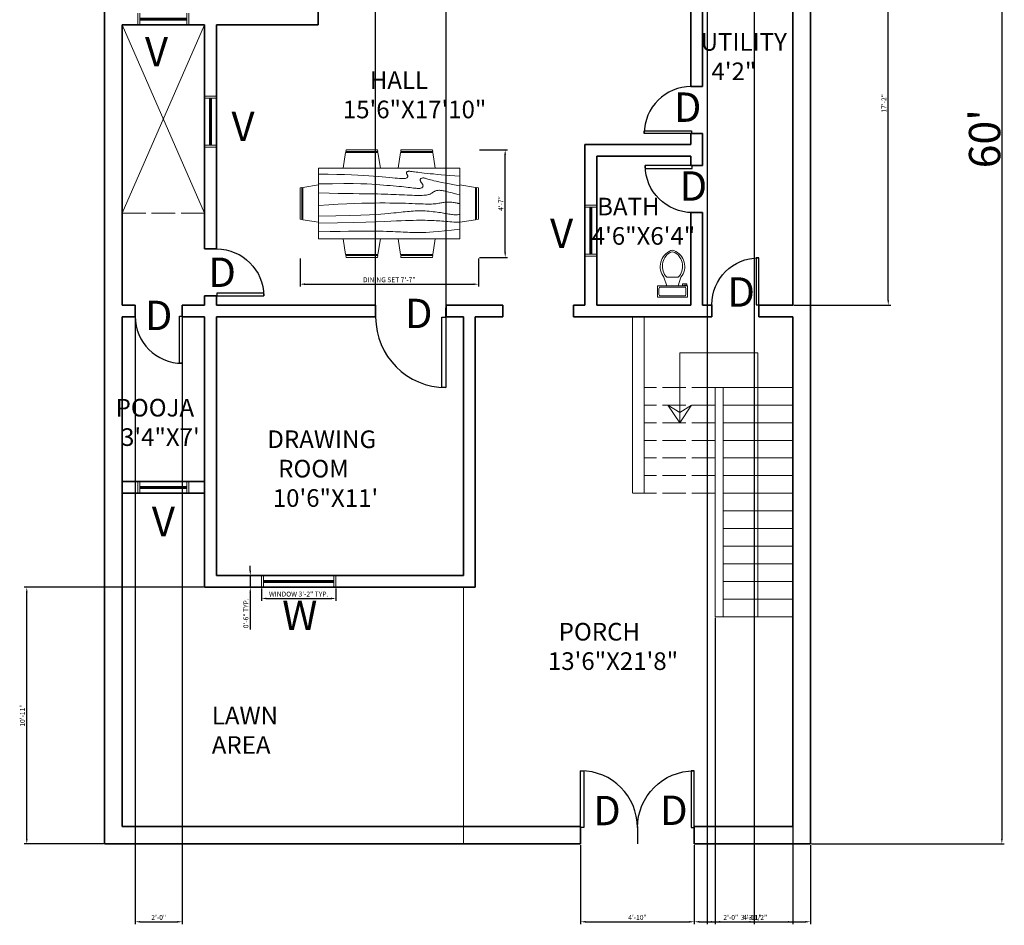
# Model space of a CAD drawing. Units: inches. Extents: x -8018 to -7514, y 7025 to 7863.
# Tile 1 of 3: x -8016 to -7514, y 7025 to 7487. Entities that reach past the tile are written whole.
import ezdxf

# ---------------------------------------------------------------- set-up
doc = ezdxf.new("R2010")
doc.units = ezdxf.units.IN
doc.linetypes.add('ACAD_ISO02W100', pattern=[15, 12, -3])
for name, color, linetype, lineweight, true_color in [('A-ANNO-DIMS', 30, 'Continuous', 18, 0xf26722), ('A-FLOR-OPEN', 41, 'Continuous', 18, 0xf4ee51), ('A-FLOR-OPEN-OVHD', 41, 'ACAD_ISO02W100', 18, 0xf4ee51), ('A-FLOR-STRS', 41, 'Continuous', 18, 0xf4ee51), ('A-FLOR-STRS-OVHD', 41, 'ACAD_ISO02W100', 18, 0xf4ee51), ('A-GLAZ', 240, 'Continuous', 18, 0xed1f24), ('A-WALL', 41, 'Continuous', 35, 0xf4ee51), ('L-SITE', 41, 'Continuous', 18, 0xf4ee51)]:
    doc.layers.add(name, color=color, linetype=linetype, lineweight=lineweight, true_color=true_color)
for name, color, linetype, lineweight in [('A-ANNO-TEXT', 7, 'Continuous', 18), ('A-AREA-IDEN', 7, 'Continuous', 18), ('A-DOOR', 4, 'Continuous', 25), ('A-FLOR-FIXT', 9, 'Continuous', 18), ('A-FURN', 9, 'Continuous', 18)]:
    doc.layers.add(name, color=color, linetype=linetype, lineweight=lineweight)
doc.styles.get("Standard").update_dxf_attribs({"font": 'arial.ttf'})
doc.dimstyles.new('ISO-25', dxfattribs={"dimtxt": 2.5, "dimasz": 2.5, "dimexe": 1.25, "dimexo": 0.625, "dimtad": 1, "dimdec": 0, "dimlunit": 3, "dimtxsty": 'Standard', "dimcen": 2.5, "dimadec": 0, "dimazin": 0, "dimtfac": 1, "dimtdec": 0, "dimtmove": 0, "dimatfit": 3, "dimfxl": 1, "dimarcsym": 0})

# ---------------------------------------------------------------- blocks, each defined once
blk = doc.blocks.new('*U8')
for p, q in [((0, 0), (0, -100)), ((750, 0), (750, -100))]:
    blk.add_line(p, q)
blk.add_lwpolyline([(0, 0), (0, 750), (43.75, 750), (43.75, 0)], close=True)
blk.add_arc((0, 0), 750, 0, 90)
blk = doc.blocks.new('Toilet - top')
for p, q in [((9.5, -6), (9.5, -2)), ((-10, -8.5), (-8, -8.5)), ((-10, -9.5), (-10, -8.5)), ((-7, -9.5), (-10, -9.5)), ((-8, -8.5), (-8, -8)), ((-7, -8), (-7, -9.5)), ((-4, -8), (-6, -14)), ((4, -8), (6, -14)), ((4, -14), (-4, -14))]:
    blk.add_line(p, q)
blk.add_lwpolyline([(10.5, -8), (10.5, 0), (-10.5, 0), (-10.5, -8)], close=True)
for points in [[(-9.5, -2), (-9.5, -6)], [(8.5, -1), (-8.5, -1)], [(-8.5, -7), (8.5, -7)]]:
    blk.add_lwpolyline(points)
for centre, radius, start, end in [((-8.62, -1.88), 0.884, 81.8699, 188.1301), ((-8.62, -6.12), 0.884, 171.8699, 278.1301), ((8.62, -1.88), 0.884, 351.8699, 98.1301), ((8.62, -6.12), 0.884, 261.8699, 8.1301), ((3.52, -21.58), 12.17, 141.46911, 247.97143), ((4.2, -21.82), 11.33, 136.36773, 238.94682), ((-3.52, -21.58), 12.17, 292.02843, 38.53071), ((-4.2, -21.82), 11.33, 301.05301, 43.63209), ((0, -27.88), 4, 245.73182, 294.26817), ((0, -29), 4, 254.86053, 285.13947)]:
    blk.add_arc(centre, radius, start, end)
blk = doc.blocks.new('Dining Set - 36 x 72 in.')
for p, q in [((-22.2343, 26.00059), (-23.4847, 17.99762)), ((-22.2304, 26), (-5.7608, 26)), ((-22, 27.5), (-22.1562, 26.50042)), ((-5.8416, 26.5), (-22.1534, 26.5)), ((-22, 27.5), (-6, 27.5)), ((-5.8437, 26.49966), (-6, 27.5)), ((-4.5152, 17.99762), (-5.7655, 25.99926)), ((5.7657, 26.00059), (4.5153, 17.99762)), ((5.7696, 26), (22.2392, 26)), ((6, 27.5), (5.8438, 26.50042)), ((22.1584, 26.5), (5.8466, 26.5)), ((6, 27.5), (22, 27.5)), ((22.1563, 26.49966), (22, 27.5)), ((23.4848, 17.99762), (22.2345, 25.99926)), ((36, 18), (-36, 18)), ((-36, 18), (-36, -18)), ((36, -18), (36, 18)), ((-45.5, 8), (-44.5004, 8.15617)), ((-45.5, 8), (-45.5, -8)), ((-44.5, -8.15843), (-44.5, 8.15338)), ((-44.0006, 8.23428), (-35.9976, 9.48474)), ((-44, 8.23041), (-44, -8.23915)), ((44.0006, 8.23428), (35.9976, 9.48474)), ((44, 8.23041), (44, -8.23915)), ((44.5, -8.15843), (44.5, 8.15338)), ((45.5, 8), (44.5005, 8.15617)), ((45.5, 8), (45.5, -8)), ((-44.4997, -8.15631), (-45.5, -8)), ((-35.9976, -9.48476), (-43.9993, -8.2345)), ((35.9976, -9.48476), (43.9993, -8.2345)), ((44.4997, -8.15631), (45.5, -8)), ((-36, -18), (36, -18)), ((-22.2343, -26.0006), (-23.4847, -17.99762)), ((-4.5152, -17.99762), (-5.7655, -25.99928)), ((5.7657, -26.0006), (4.5153, -17.99762)), ((23.4848, -17.99762), (22.2345, -25.99928)), ((-22.2304, -26), (-5.7608, -26)), ((-22, -27.5), (-22.1562, -26.50044)), ((-5.8416, -26.5), (-22.1534, -26.5)), ((-22, -27.5), (-6, -27.5)), ((-5.8437, -26.49967), (-6, -27.5)), ((5.7696, -26), (22.2392, -26)), ((6, -27.5), (5.8438, -26.50044)), ((22.1584, -26.5), (5.8466, -26.5)), ((6, -27.5), (22, -27.5)), ((22.1563, -26.49967), (22, -27.5))]:
    blk.add_line(p, q)
for points in [[(-36, 15), (-31.1772, 14.97754), (-26.8079, 14.91406), (-22.8538, 14.81543), (-19.276, 14.6875), (-16.0362, 14.53613), (-13.0957, 14.36718), (-10.4159, 14.18652), (-7.9583, 14), (-5.6904, 13.81315), (-3.6035, 13.63021), (-1.6954, 13.45508), (0.0365, 13.29166), (1.5945, 13.14388), (2.9811, 13.01562), (4.1988, 12.9108), (5.25, 12.83333), (6.1393, 12.78613), (6.8802, 12.76823), (7.4883, 12.77767), (7.9792, 12.8125), (8.3685, 12.87077), (8.6719, 12.95052), (8.9049, 13.0498), (9.0833, 13.16666), (9.2205, 13.29899), (9.3216, 13.44401), (9.3895, 13.59879), (9.4271, 13.76041), (9.4373, 13.92594), (9.4232, 14.09245), (9.3875, 14.257), (9.3333, 14.41666), (9.2638, 14.56917), (9.1836, 14.71484), (9.0975, 14.85465), (9.0104, 14.98958), (8.9272, 15.1206), (8.8529, 15.2487), (8.7922, 15.37483), (8.75, 15.5), (8.7305, 15.62467), (8.7344, 15.74739), (8.7617, 15.86621), (8.8125, 15.97916), (8.8867, 16.08431), (8.9844, 16.17968), (9.1055, 16.26334), (9.25, 16.33333), (9.4189, 16.38802), (9.6172, 16.42708), (9.8506, 16.45052), (10.125, 16.45833), (10.4463, 16.45052), (10.8203, 16.42708), (11.2529, 16.38802), (11.75, 16.33333), (12.3184, 16.26318), (12.9694, 16.17838), (13.7151, 16.07991), (14.5677, 15.96875), (15.5395, 15.84586), (16.6426, 15.71224), (17.8893, 15.56884), (19.2917, 15.41666), (20.859, 15.25667), (22.5879, 15.08984), (24.4721, 14.91715), (26.5052, 14.73958), (28.6809, 14.5581), (30.9929, 14.3737), (33.4347, 14.18733), (36, 14)], [(-36, 10), (-28.9766, 10.14274), (-23.1725, 10.20442), (-18.4241, 10.19775), (-14.5677, 10.13541), (-11.4399, 10.03011), (-8.877, 9.89453), (-6.7154, 9.74137), (-4.7917, 9.58333), (-2.9698, 9.43082), (-1.2246, 9.28515), (0.4415, 9.14534), (2.026, 9.01041), (3.5266, 8.87939), (4.9408, 8.7513), (6.266, 8.62516), (7.5, 8.5), (8.6411, 8.37549), (9.6914, 8.2539), (10.6538, 8.13818), (11.5312, 8.03125), (12.3267, 7.93603), (13.043, 7.85547), (13.6831, 7.79248), (14.25, 7.75), (14.7471, 7.7303), (15.1797, 7.73307), (15.5537, 7.75732), (15.875, 7.80208), (16.1494, 7.86637), (16.3828, 7.94922), (16.5811, 8.04964), (16.75, 8.16666), (16.8944, 8.29915), (17.0143, 8.44531), (17.1089, 8.60319), (17.1771, 8.77083), (17.218, 8.94629), (17.2305, 9.1276), (17.2137, 9.31282), (17.1667, 9.5), (17.0895, 9.6875), (16.987, 9.875), (16.8649, 10.0625), (16.7292, 10.25), (16.5856, 10.4375), (16.4401, 10.625), (16.2985, 10.8125), (16.1667, 11), (16.05, 11.18733), (15.9518, 11.3737), (15.8752, 11.5581), (15.8229, 11.73958), (15.798, 11.91715), (15.8034, 12.08984), (15.842, 12.25667), (15.9167, 12.41666), (16.0295, 12.56836), (16.1784, 12.70833), (16.3605, 12.83268), (16.5729, 12.9375), (16.8127, 13.01888), (17.0768, 13.07291), (17.3625, 13.0957), (17.6667, 13.08333), (17.9894, 13.03312), (18.3418, 12.94726), (18.7382, 12.82918), (19.1927, 12.68229), (19.7195, 12.51001), (20.3327, 12.31575), (21.0465, 12.10294), (21.875, 11.875), (22.8357, 11.63354), (23.959, 11.37304), (25.2786, 11.08618), (26.8282, 10.76562), (28.6414, 10.40405), (30.752, 9.99414), (33.1936, 9.52856), (36, 9)], [(-36, 5.5), (-30.7157, 5.3348), (-26.069, 5.20963), (-21.9946, 5.11767), (-18.4271, 5.05208), (-15.3009, 5.00602), (-12.5508, 4.97265), (-10.1112, 4.94515), (-7.9167, 4.91666), (-5.909, 4.88167), (-4.0586, 4.83984), (-2.3429, 4.79215), (-0.7396, 4.73958), (0.7739, 4.6831), (2.22, 4.6237), (3.6213, 4.56233), (5, 4.5), (6.373, 4.43782), (7.7344, 4.3776), (9.0723, 4.32129), (10.375, 4.27083), (11.6309, 4.22819), (12.8281, 4.19531), (13.9551, 4.17415), (15, 4.16666), (15.954, 4.17448), (16.819, 4.19791), (17.6001, 4.23698), (18.3021, 4.29166), (18.9299, 4.36198), (19.4883, 4.44791), (19.9823, 4.54948), (20.4167, 4.66666), (20.7969, 4.79899), (21.1302, 4.94401), (21.4245, 5.09879), (21.6875, 5.26041), (21.9271, 5.42594), (22.1511, 5.59245), (22.3672, 5.757), (22.5834, 5.91666), (22.8065, 6.06868), (23.0404, 6.21093), (23.2879, 6.34147), (23.5521, 6.45833), (23.8358, 6.55957), (24.142, 6.64323), (24.4735, 6.70735), (24.8334, 6.75), (25.2235, 6.76969), (25.642, 6.76692), (26.0858, 6.74267), (26.5521, 6.69791), (27.0379, 6.63362), (27.5404, 6.55078), (28.0565, 6.45036), (28.5834, 6.33333), (29.1242, 6.19987), (29.7071, 6.04687), (30.3661, 5.87044), (31.1354, 5.66666), (32.0493, 5.43164), (33.142, 5.16146), (34.4475, 4.85221), (36, 4.5)], [(-36, -1), (-30.7915, -0.6591), (-26.0195, -0.38216), (-21.6519, -0.16284), (-17.6563, 0.00521), (-14.0005, 0.12833), (-10.6523, 0.21289), (-7.5796, 0.26522), (-4.75, 0.29166), (-2.134, 0.29793), (0.2878, 0.28711), (2.5317, 0.26163), (4.6146, 0.22396), (6.5529, 0.17651), (8.3633, 0.12174), (10.0623, 0.06209), (11.6667, 0), (13.1899, -0.06201), (14.6341, -0.1211), (15.9982, -0.17432), (17.2813, -0.21875), (18.4823, -0.25147), (19.6003, -0.26953), (20.6343, -0.27002), (21.5834, -0.25), (22.4481, -0.20768), (23.2357, -0.14584), (23.9549, -0.06836), (24.6146, 0.02083), (25.2235, 0.11784), (25.7904, 0.21875), (26.3241, 0.31966), (26.8334, 0.41666), (27.3265, 0.50618), (27.8099, 0.58593), (28.2894, 0.65397), (28.7709, 0.70833), (29.2601, 0.74707), (29.763, 0.76823), (30.2855, 0.76985), (30.8334, 0.75), (31.4088, 0.70784), (31.9994, 0.64713), (32.589, 0.57275), (33.1615, 0.48958), (33.7008, 0.4025), (34.1908, 0.3164), (34.6153, 0.23616), (34.9584, 0.16666), (35.2099, 0.11165), (35.3848, 0.07031), (35.504, 0.04069), (35.5886, 0.02083), (35.6594, 0.00879), (35.7377, 0.0026), (35.8442, 0.00032), (36, 0)], [(-36, -6.5), (-27.1843, -6.31267), (-20.084, -6.1263), (-14.469, -5.9419), (-10.1094, -5.76042), (-6.7752, -5.58285), (-4.2363, -5.41016), (-2.2629, -5.24333), (-0.625, -5.08334), (0.8708, -4.93099), (2.2715, -4.78646), (3.5872, -4.64974), (4.8281, -4.52084), (6.0046, -4.39974), (7.127, -4.28646), (8.2053, -4.18099), (9.25, -4.08334), (10.2705, -3.99382), (11.2734, -3.91407), (12.2647, -3.84603), (13.25, -3.79167), (14.2354, -3.75293), (15.2266, -3.73177), (16.2295, -3.73015), (17.25, -3.75), (18.2912, -3.79248), (19.3451, -3.85547), (20.4009, -3.93604), (21.4479, -4.03125), (22.4754, -4.13819), (23.4727, -4.25391), (24.4289, -4.37549), (25.3334, -4.5), (26.1785, -4.62492), (26.9694, -4.74935), (27.7145, -4.87281), (28.4219, -4.99479), (29.1, -5.11483), (29.7572, -5.23242), (30.4016, -5.34709), (31.0417, -5.45834), (31.6837, -5.56437), (32.3262, -5.65821), (32.9658, -5.73153), (33.599, -5.77604), (34.2224, -5.78345), (34.8327, -5.74545), (35.4264, -5.65373), (36, -5.5)], [(-36, -10), (-26.4022, -9.81299), (-18.4675, -9.62891), (-11.9839, -9.45069), (-6.7396, -9.28125), (-2.5226, -9.12354), (0.8789, -8.98047), (3.6769, -8.85498), (6.0833, -8.75), (8.2767, -8.66765), (10.3021, -8.60677), (12.1712, -8.56543), (13.8958, -8.54167), (15.4876, -8.53353), (16.9583, -8.53907), (18.3197, -8.55632), (19.5834, -8.58334), (20.7616, -8.61841), (21.8685, -8.66081), (22.9188, -8.71004), (23.9271, -8.76563), (24.9081, -8.82707), (25.8763, -8.89388), (26.8465, -8.96558), (27.8334, -9.04167), (28.8474, -9.12118), (29.8828, -9.20117), (30.93, -9.27824), (31.9792, -9.34896), (33.0205, -9.40991), (34.0443, -9.45768), (35.0407, -9.48885), (36, -9.5)], [(-36, -14.5), (-30.0881, -14.33513), (-25.0332, -14.21224), (-20.7312, -14.12647), (-17.0781, -14.07292), (-13.97, -14.04671), (-11.3027, -14.04297), (-8.9724, -14.05681), (-6.875, -14.08334), (-4.9224, -14.11833), (-3.0905, -14.16016), (-1.3709, -14.20785), (0.2448, -14.26042), (1.7647, -14.3169), (3.1973, -14.3763), (4.5507, -14.43767), (5.8333, -14.5), (7.0554, -14.5621), (8.235, -14.62175), (9.3922, -14.67652), (10.5469, -14.72396), (11.7192, -14.76164), (12.929, -14.78711), (14.1965, -14.79794), (15.5417, -14.79167), (16.9933, -14.76424), (18.6152, -14.70508), (20.4804, -14.60197), (22.6615, -14.44271), (25.2312, -14.21509), (28.2624, -13.9069), (31.8277, -13.50594), (36, -13)]]:
    blk.add_lwpolyline(points)
blk = doc.blocks.new('*D107')
at = {"layer": 'A-ANNO-DIMS', "color": 0, "lineweight": -2, "transparency": 16777216}
for p, q in [((-7612.17, 7786.37), (-7513.89, 7786.37)), ((-7515.14, 7783.87), (-7515.14, 7068.87)), ((-7612.17, 7066.37), (-7513.89, 7066.37))]:
    blk.add_line(p, q, dxfattribs=at)
at = {"layer": 'A-ANNO-DIMS', "color": 0, "transparency": 16777216}
for points in [[(-7515.56, 7783.87), (-7514.73, 7783.87), (-7515.14, 7786.37)], [(-7515.56, 7068.87), (-7514.73, 7068.87), (-7515.14, 7066.37)]]:
    blk.add_solid(points, dxfattribs=at)
at = {"layer": 'Defpoints', "color": 0, "transparency": 16777216}
for p in [(-7612.8, 7786.37), (-7612.8, 7066.37), (-7515.14, 7066.37)]:
    blk.add_point(p, dxfattribs=at)
at = {"layer": 'A-ANNO-DIMS', "color": 0, "transparency": 16777216, "insert": (-7523.94, 7426.37), "char_height": 2.5, "attachment_point": 5, "rotation": 90}
blk.add_mtext("{\\H6.4x;60'}", dxfattribs=at)
blk = doc.blocks.new('VENT-24IN-6IN-WALL')
for p, q in [((0, 26), (6, 26)), ((0, 25), (6, 25)), ((2.5, 1), (2.5, 25)), ((3, 1), (3, 25)), ((3.5, 1), (3.5, 25)), ((0, 1), (6, 1)), ((0, 0), (6, 0))]:
    blk.add_line(p, q)
blk = doc.blocks.new('WINDOW-36IN-6IN-WALL')
for p, q in [((0, 38), (6, 38)), ((0, 37), (6, 37)), ((2.5, 1), (2.5, 37)), ((3, 1), (3, 37)), ((3.5, 1), (3.5, 37)), ((0, 1), (6, 1)), ((0, 0), (6, 0))]:
    blk.add_line(p, q)
blk = doc.blocks.new('*D114')
at = {"layer": 'A-ANNO-DIMS', "color": 0, "lineweight": -2, "transparency": 16777216}
for p, q in [((-7892.8, 7196.74), (-7892.8, 7190.42)), ((-7854.8, 7196.74), (-7854.8, 7190.42)), ((-7890.3, 7191.67), (-7857.3, 7191.67))]:
    blk.add_line(p, q, dxfattribs=at)
at = {"layer": 'A-ANNO-DIMS', "color": 0, "transparency": 16777216}
for points in [[(-7890.3, 7192.08), (-7890.3, 7191.25), (-7892.8, 7191.67)], [(-7857.3, 7192.08), (-7857.3, 7191.25), (-7854.8, 7191.67)]]:
    blk.add_solid(points, dxfattribs=at)
at = {"layer": 'Defpoints', "color": 0, "transparency": 16777216}
for p in [(-7892.8, 7197.37), (-7854.8, 7197.37), (-7854.8, 7191.67)]:
    blk.add_point(p, dxfattribs=at)
at = {"layer": 'A-ANNO-DIMS', "color": 0, "transparency": 16777216, "insert": (-7873.8, 7193.59), "char_height": 2.5, "attachment_point": 5}
blk.add_mtext('WINDOW 3\'-2" TYP.', dxfattribs=at)
blk = doc.blocks.new('*D115')
at = {"layer": 'A-ANNO-DIMS', "color": 0, "lineweight": -2, "transparency": 16777216}
for p, q in [((-7898.5, 7205.87), (-7898.5, 7208.37)), ((-7893.42, 7203.37), (-7899.75, 7203.37)), ((-7898.5, 7203.37), (-7898.5, 7197.37)), ((-7893.42, 7197.37), (-7899.75, 7197.37)), ((-7898.5, 7194.87), (-7898.5, 7175.88))]:
    blk.add_line(p, q, dxfattribs=at)
at = {"layer": 'A-ANNO-DIMS', "color": 0, "transparency": 16777216}
for points in [[(-7898.92, 7205.87), (-7898.08, 7205.87), (-7898.5, 7203.37)], [(-7898.92, 7194.87), (-7898.08, 7194.87), (-7898.5, 7197.37)]]:
    blk.add_solid(points, dxfattribs=at)
at = {"layer": 'Defpoints', "color": 0, "transparency": 16777216}
for p in [(-7892.8, 7203.37), (-7898.5, 7197.37), (-7892.8, 7197.37)]:
    blk.add_point(p, dxfattribs=at)
at = {"layer": 'A-ANNO-DIMS', "color": 0, "transparency": 16777216, "insert": (-7900.4, 7184.12), "char_height": 2.5, "attachment_point": 5, "rotation": 90}
blk.add_mtext('0\'-6" TYP.', dxfattribs=at)
blk = doc.blocks.new('*D128')
at = {"layer": 'A-ANNO-DIMS', "color": 0, "lineweight": -2, "transparency": 16777216}
for p, q in [((-7873.12, 7365.11), (-7873.12, 7350.83)), ((-7782.12, 7365.11), (-7782.12, 7350.83)), ((-7870.62, 7352.08), (-7784.62, 7352.08))]:
    blk.add_line(p, q, dxfattribs=at)
at = {"layer": 'A-ANNO-DIMS', "color": 0, "transparency": 16777216}
for points in [[(-7870.62, 7352.5), (-7870.62, 7351.67), (-7873.12, 7352.08)], [(-7784.62, 7352.5), (-7784.62, 7351.67), (-7782.12, 7352.08)]]:
    blk.add_solid(points, dxfattribs=at)
at = {"layer": 'Defpoints', "color": 0, "transparency": 16777216}
for p in [(-7873.12, 7365.73), (-7782.12, 7365.73), (-7782.12, 7352.08)]:
    blk.add_point(p, dxfattribs=at)
at = {"layer": 'A-ANNO-DIMS', "color": 0, "transparency": 16777216, "insert": (-7827.62, 7354), "char_height": 2.5, "attachment_point": 5}
blk.add_mtext('DINING SET 7\'-7"', dxfattribs=at)
blk = doc.blocks.new('*D129')
at = {"layer": 'A-ANNO-DIMS', "color": 0, "lineweight": -2, "transparency": 16777216}
for p, q in [((-7781.5, 7420.73), (-7767.22, 7420.73)), ((-7768.47, 7368.23), (-7768.47, 7418.23)), ((-7781.5, 7365.73), (-7767.22, 7365.73))]:
    blk.add_line(p, q, dxfattribs=at)
at = {"layer": 'A-ANNO-DIMS', "color": 0, "transparency": 16777216}
for points in [[(-7768.89, 7418.23), (-7768.06, 7418.23), (-7768.47, 7420.73)], [(-7768.89, 7368.23), (-7768.06, 7368.23), (-7768.47, 7365.73)]]:
    blk.add_solid(points, dxfattribs=at)
at = {"layer": 'Defpoints', "color": 0, "transparency": 16777216}
for p in [(-7782.12, 7420.73), (-7768.47, 7420.73), (-7782.12, 7365.73)]:
    blk.add_point(p, dxfattribs=at)
at = {"layer": 'A-ANNO-DIMS', "color": 0, "transparency": 16777216, "insert": (-7770.35, 7393.23), "char_height": 2.5, "attachment_point": 5, "rotation": 90}
blk.add_mtext('4\'-7"', dxfattribs=at)
blk = doc.blocks.new('*D130')
at = {"layer": 'A-ANNO-DIMS', "color": 0, "lineweight": -2, "transparency": 16777216}
for p, q in [((-7730, 7065.74), (-7730, 7025.42)), ((-7672, 7065.74), (-7672, 7025.42)), ((-7727.5, 7026.67), (-7674.5, 7026.67))]:
    blk.add_line(p, q, dxfattribs=at)
at = {"layer": 'A-ANNO-DIMS', "color": 0, "transparency": 16777216}
for points in [[(-7727.5, 7027.08), (-7727.5, 7026.25), (-7730, 7026.67)], [(-7674.5, 7027.08), (-7674.5, 7026.25), (-7672, 7026.67)]]:
    blk.add_solid(points, dxfattribs=at)
at = {"layer": 'Defpoints', "color": 0, "transparency": 16777216}
for p in [(-7730, 7066.37), (-7672, 7066.37), (-7672, 7026.67)]:
    blk.add_point(p, dxfattribs=at)
at = {"layer": 'A-ANNO-DIMS', "color": 0, "transparency": 16777216, "insert": (-7701, 7028.57), "char_height": 2.5, "attachment_point": 5}
blk.add_mtext('4\'-10"', dxfattribs=at)
blk = doc.blocks.new('*D131')
at = {"layer": 'A-ANNO-DIMS', "color": 0, "lineweight": -2, "transparency": 16777216}
for p, q in [((-7672, 7065.74), (-7672, 7025.42)), ((-7612.8, 7065.74), (-7612.8, 7025.42)), ((-7669.5, 7026.67), (-7615.3, 7026.67))]:
    blk.add_line(p, q, dxfattribs=at)
at = {"layer": 'A-ANNO-DIMS', "color": 0, "transparency": 16777216}
for points in [[(-7669.5, 7027.08), (-7669.5, 7026.25), (-7672, 7026.67)], [(-7615.3, 7027.08), (-7615.3, 7026.25), (-7612.8, 7026.67)]]:
    blk.add_solid(points, dxfattribs=at)
at = {"layer": 'Defpoints', "color": 0, "transparency": 16777216}
for p in [(-7672, 7066.37), (-7612.8, 7066.37), (-7612.8, 7026.67)]:
    blk.add_point(p, dxfattribs=at)
at = {"layer": 'A-ANNO-DIMS', "color": 0, "transparency": 16777216, "insert": (-7642.4, 7028.55), "char_height": 2.5, "attachment_point": 5}
blk.add_mtext('4\'-11"', dxfattribs=at)
blk = doc.blocks.new('*D132')
at = {"layer": 'A-ANNO-DIMS', "color": 0, "lineweight": -2, "transparency": 16777216}
for p, q in [((-7621.17, 7547.37), (-7571.85, 7547.37)), ((-7573.1, 7343.87), (-7573.1, 7544.87)), ((-7621.17, 7341.37), (-7571.85, 7341.37))]:
    blk.add_line(p, q, dxfattribs=at)
at = {"layer": 'A-ANNO-DIMS', "color": 0, "transparency": 16777216}
for points in [[(-7573.52, 7544.87), (-7572.68, 7544.87), (-7573.1, 7547.37)], [(-7573.52, 7343.87), (-7572.68, 7343.87), (-7573.1, 7341.37)]]:
    blk.add_solid(points, dxfattribs=at)
at = {"layer": 'Defpoints', "color": 0, "transparency": 16777216}
for p in [(-7621.8, 7547.37), (-7573.1, 7547.37), (-7621.8, 7341.37)]:
    blk.add_point(p, dxfattribs=at)
at = {"layer": 'A-ANNO-DIMS', "color": 0, "transparency": 16777216, "insert": (-7574.98, 7444.37), "char_height": 2.5, "attachment_point": 5, "rotation": 90}
blk.add_mtext('17\'-2"', dxfattribs=at)
blk = doc.blocks.new('*D133')
at = {"layer": 'A-ANNO-DIMS', "color": 0, "lineweight": -2, "transparency": 16777216}
for p, q in [((-7834.62, 7335.99), (-7834.62, 7827.32)), ((-7832.12, 7826.07), (-7801.12, 7826.07)), ((-7798.62, 7335.99), (-7798.62, 7827.32))]:
    blk.add_line(p, q, dxfattribs=at)
at = {"layer": 'A-ANNO-DIMS', "color": 0, "transparency": 16777216}
for points in [[(-7832.12, 7826.48), (-7832.12, 7825.65), (-7834.62, 7826.07)], [(-7801.12, 7826.48), (-7801.12, 7825.65), (-7798.62, 7826.07)]]:
    blk.add_solid(points, dxfattribs=at)
at = {"layer": 'Defpoints', "color": 0, "transparency": 16777216}
for p in [(-7798.62, 7826.07), (-7834.62, 7335.37), (-7798.62, 7335.37)]:
    blk.add_point(p, dxfattribs=at)
at = {"layer": 'A-ANNO-DIMS', "color": 0, "transparency": 16777216, "insert": (-7816.62, 7827.97), "char_height": 2.5, "attachment_point": 5}
blk.add_mtext('3\'-0"', dxfattribs=at)
blk = doc.blocks.new('*D134')
at = {"layer": 'A-ANNO-DIMS', "color": 0, "lineweight": -2, "transparency": 16777216}
for p, q in [((-7957.2, 7334.74), (-7957.2, 7025.42)), ((-7933.2, 7334.74), (-7933.2, 7025.42)), ((-7954.7, 7026.67), (-7935.7, 7026.67))]:
    blk.add_line(p, q, dxfattribs=at)
at = {"layer": 'A-ANNO-DIMS', "color": 0, "transparency": 16777216}
for points in [[(-7954.7, 7027.08), (-7954.7, 7026.25), (-7957.2, 7026.67)], [(-7935.7, 7027.08), (-7935.7, 7026.25), (-7933.2, 7026.67)]]:
    blk.add_solid(points, dxfattribs=at)
at = {"layer": 'Defpoints', "color": 0, "transparency": 16777216}
for p in [(-7957.2, 7335.37), (-7933.2, 7335.37), (-7933.2, 7026.67)]:
    blk.add_point(p, dxfattribs=at)
at = {"layer": 'A-ANNO-DIMS', "color": 0, "transparency": 16777216, "insert": (-7945.2, 7028.57), "char_height": 2.5, "attachment_point": 5}
blk.add_mtext('2\'-0"', dxfattribs=at)
blk = doc.blocks.new('*D135')
at = {"layer": 'A-ANNO-DIMS', "color": 0, "lineweight": -2, "transparency": 16777216}
for p, q in [((-7922.42, 7197.37), (-8013.75, 7197.37)), ((-8012.5, 7068.87), (-8012.5, 7194.87)), ((-7973.42, 7066.37), (-8013.75, 7066.37))]:
    blk.add_line(p, q, dxfattribs=at)
at = {"layer": 'A-ANNO-DIMS', "color": 0, "transparency": 16777216}
for points in [[(-8012.92, 7194.87), (-8012.08, 7194.87), (-8012.5, 7197.37)], [(-8012.92, 7068.87), (-8012.08, 7068.87), (-8012.5, 7066.37)]]:
    blk.add_solid(points, dxfattribs=at)
at = {"layer": 'Defpoints', "color": 0, "transparency": 16777216}
for p in [(-8012.5, 7197.37), (-7921.8, 7197.37), (-7972.8, 7066.37)]:
    blk.add_point(p, dxfattribs=at)
at = {"layer": 'A-ANNO-DIMS', "color": 0, "transparency": 16777216, "insert": (-8014.4, 7131.87), "char_height": 2.5, "attachment_point": 5, "rotation": 90}
blk.add_mtext('10\'-11"', dxfattribs=at)
blk = doc.blocks.new('*D136')
at = {"layer": 'A-ANNO-DIMS', "color": 0, "lineweight": -2, "transparency": 16777216}
for p, q in [((-7661.3, 7181.74), (-7661.3, 7025.42)), ((-7621.8, 7181.74), (-7621.8, 7025.42)), ((-7658.8, 7026.67), (-7624.3, 7026.67))]:
    blk.add_line(p, q, dxfattribs=at)
at = {"layer": 'A-ANNO-DIMS', "color": 0, "transparency": 16777216}
for points in [[(-7658.8, 7027.08), (-7658.8, 7026.25), (-7661.3, 7026.67)], [(-7624.3, 7027.08), (-7624.3, 7026.25), (-7621.8, 7026.67)]]:
    blk.add_solid(points, dxfattribs=at)
at = {"layer": 'Defpoints', "color": 0, "transparency": 16777216}
for p in [(-7661.3, 7182.37), (-7621.8, 7182.37), (-7621.8, 7026.67)]:
    blk.add_point(p, dxfattribs=at)
at = {"layer": 'A-ANNO-DIMS', "color": 0, "transparency": 16777216, "insert": (-7641.55, 7028.58), "char_height": 2.5, "attachment_point": 5}
blk.add_mtext('3\'-3 1/2"', dxfattribs=at)
blk = doc.blocks.new('*D137')
at = {"layer": 'A-ANNO-DIMS', "color": 0, "lineweight": -2, "transparency": 16777216}
for p, q in [((-7665.42, 7686.74), (-7665.42, 7025.42)), ((-7641.42, 7686.74), (-7641.42, 7025.42)), ((-7662.92, 7026.67), (-7643.92, 7026.67))]:
    blk.add_line(p, q, dxfattribs=at)
at = {"layer": 'A-ANNO-DIMS', "color": 0, "transparency": 16777216}
for points in [[(-7662.92, 7027.08), (-7662.92, 7026.25), (-7665.42, 7026.67)], [(-7643.92, 7027.08), (-7643.92, 7026.25), (-7641.42, 7026.67)]]:
    blk.add_solid(points, dxfattribs=at)
at = {"layer": 'Defpoints', "color": 0, "transparency": 16777216}
for p in [(-7665.42, 7687.37), (-7641.42, 7687.37), (-7641.42, 7026.67)]:
    blk.add_point(p, dxfattribs=at)
at = {"layer": 'A-ANNO-DIMS', "color": 0, "transparency": 16777216, "insert": (-7653.42, 7028.57), "char_height": 2.5, "attachment_point": 5}
blk.add_mtext('2\'-0"', dxfattribs=at)

msp = doc.modelspace()

# ---------------------------------------------------------------- linework, layer by layer
at = {"layer": 'A-DOOR'}
msp.add_line((-7701, 7075.37), (-7701, 7066.37), dxfattribs=at)
at = {"layer": 'A-FLOR-OPEN'}
for p, q in [((-7963.8, 7388.37), (-7921.8, 7484.37)), ((-7963.8, 7484.37), (-7921.8, 7388.37))]:
    msp.add_line(p, q, dxfattribs=at)
at = {"layer": 'A-FLOR-OPEN-OVHD'}
msp.add_line((-7963.8, 7388.37), (-7921.8, 7388.37), dxfattribs=at)
at = {"layer": 'A-FLOR-STRS'}
for p, q in [((-7703.52, 7335.37), (-7703.52, 7245.37)), ((-7697.52, 7335.37), (-7697.52, 7245.37)), ((-7679.41, 7281.37), (-7679.41, 7317.06)), ((-7679.41, 7317.06), (-7639.55, 7317.06)), ((-7639.55, 7317.06), (-7639.55, 7182.37)), ((-7621.8, 7299.37), (-7661.3, 7299.37)), ((-7661.3, 7299.37), (-7661.3, 7182.37)), ((-7657.3, 7299.37), (-7657.3, 7182.37)), ((-7679.41, 7286.56), (-7685.46, 7290.37)), ((-7685.46, 7290.37), (-7679.41, 7281.37)), ((-7679.41, 7281.37), (-7673.49, 7290.37)), ((-7673.49, 7290.37), (-7679.41, 7286.56)), ((-7679.41, 7281.37), (-7679.41, 7289.93)), ((-7621.8, 7290.37), (-7657.3, 7290.37)), ((-7621.8, 7281.37), (-7657.3, 7281.37)), ((-7621.8, 7272.37), (-7657.3, 7272.37)), ((-7621.8, 7263.37), (-7657.3, 7263.37)), ((-7621.8, 7254.37), (-7657.3, 7254.37)), ((-7621.8, 7245.37), (-7657.3, 7245.37)), ((-7621.8, 7236.37), (-7657.3, 7236.37)), ((-7621.8, 7227.37), (-7657.3, 7227.37)), ((-7621.8, 7218.37), (-7657.3, 7218.37)), ((-7621.8, 7209.37), (-7657.3, 7209.37)), ((-7621.8, 7200.37), (-7657.3, 7200.37)), ((-7621.8, 7191.37), (-7657.3, 7191.37)), ((-7621.8, 7182.37), (-7661.3, 7182.37))]:
    msp.add_line(p, q, dxfattribs=at)
at = {"layer": 'A-FLOR-STRS-OVHD'}
for p, q in [((-7661.3, 7299.37), (-7697.52, 7299.37)), ((-7661.3, 7290.37), (-7697.52, 7290.37)), ((-7661.3, 7281.37), (-7697.52, 7281.37)), ((-7661.3, 7272.37), (-7697.52, 7272.37)), ((-7661.3, 7263.37), (-7697.52, 7263.37)), ((-7661.3, 7254.37), (-7697.52, 7254.37)), ((-7661.3, 7245.37), (-7703.52, 7245.37))]:
    msp.add_line(p, q, dxfattribs=at)
at = {"layer": 'A-WALL'}
for p, q in [((-7972.8, 7066.37), (-7972.8, 7786.37)), ((-7612.8, 7786.37), (-7612.8, 7066.37)), ((-7863.8, 7484.37), (-7863.8, 7587.95)), ((-7667.8, 7547.37), (-7667.8, 7452.92)), ((-7621.8, 7547.37), (-7621.8, 7341.37)), ((-7673.8, 7493.37), (-7673.8, 7452.92)), ((-7963.8, 7484.37), (-7921.8, 7484.37)), ((-7963.8, 7341.37), (-7963.8, 7484.37)), ((-7921.8, 7484.37), (-7921.8, 7370.1)), ((-7915.8, 7484.37), (-7915.8, 7370.1)), ((-7915.8, 7484.37), (-7863.8, 7484.37)), ((-7673.8, 7452.92), (-7667.8, 7452.92)), ((-7673.8, 7428.92), (-7667.8, 7428.92)), ((-7673.8, 7428.92), (-7673.8, 7423.37)), ((-7667.8, 7428.92), (-7667.8, 7412.6)), ((-7673.8, 7423.37), (-7727.8, 7423.37)), ((-7727.8, 7423.37), (-7727.8, 7341.37)), ((-7673.8, 7417.37), (-7721.8, 7417.37)), ((-7721.8, 7417.37), (-7721.8, 7341.37)), ((-7673.8, 7417.37), (-7673.8, 7412.6)), ((-7673.8, 7388.6), (-7673.8, 7341.37)), ((-7667.8, 7388.6), (-7667.8, 7341.37)), ((-7921.8, 7370.1), (-7915.8, 7370.1)), ((-7921.8, 7346.1), (-7915.8, 7346.1)), ((-7921.8, 7346.1), (-7921.8, 7341.37)), ((-7915.8, 7346.1), (-7915.8, 7341.37)), ((-7957.2, 7341.37), (-7963.8, 7341.37)), ((-7957.2, 7341.37), (-7957.2, 7335.37)), ((-7921.8, 7341.37), (-7933.2, 7341.37)), ((-7933.2, 7341.37), (-7933.2, 7335.37)), ((-7834.62, 7341.37), (-7915.8, 7341.37)), ((-7834.62, 7335.37), (-7834.62, 7341.37)), ((-7798.62, 7335.37), (-7798.62, 7341.37)), ((-7769.64, 7341.37), (-7798.62, 7341.37)), ((-7769.64, 7341.37), (-7769.64, 7335.37)), ((-7727.8, 7341.37), (-7733.64, 7341.37)), ((-7733.64, 7341.37), (-7733.64, 7335.37)), ((-7673.8, 7341.37), (-7721.8, 7341.37)), ((-7663.08, 7341.37), (-7667.8, 7341.37)), ((-7663.08, 7341.37), (-7663.08, 7335.37)), ((-7621.8, 7341.37), (-7639.08, 7341.37)), ((-7639.08, 7341.37), (-7639.08, 7335.37)), ((-7963.8, 7197.37), (-7963.8, 7335.37)), ((-7957.2, 7335.37), (-7963.8, 7335.37)), ((-7921.8, 7335.37), (-7933.2, 7335.37)), ((-7921.8, 7335.37), (-7921.8, 7197.37)), ((-7915.8, 7335.37), (-7915.8, 7203.37)), ((-7834.62, 7335.37), (-7915.8, 7335.37)), ((-7789.8, 7335.37), (-7798.62, 7335.37)), ((-7789.8, 7335.37), (-7789.8, 7203.37)), ((-7783.8, 7335.37), (-7783.8, 7197.37)), ((-7769.64, 7335.37), (-7783.8, 7335.37)), ((-7703.52, 7335.37), (-7733.64, 7335.37)), ((-7663.08, 7335.37), (-7703.52, 7335.37)), ((-7621.8, 7335.37), (-7639.08, 7335.37)), ((-7621.8, 7335.37), (-7621.8, 7075.37)), ((-7921.8, 7251.37), (-7963.8, 7251.37)), ((-7921.8, 7245.37), (-7963.8, 7245.37)), ((-7789.8, 7203.37), (-7915.8, 7203.37)), ((-7963.8, 7075.37), (-7963.8, 7197.37)), ((-7783.8, 7197.37), (-7921.8, 7197.37)), ((-7730, 7075.37), (-7963.8, 7075.37)), ((-7730, 7075.37), (-7730, 7066.37)), ((-7621.8, 7075.37), (-7672, 7075.37)), ((-7672, 7075.37), (-7672, 7066.37)), ((-7730, 7066.37), (-7972.8, 7066.37)), ((-7612.8, 7066.37), (-7672, 7066.37))]:
    msp.add_line(p, q, dxfattribs=at)
for points in [[(-7673.8, 7412.6), (-7667.8, 7412.6)], [(-7673.8, 7388.6), (-7667.8, 7388.6)]]:
    msp.add_lwpolyline(points, dxfattribs=at)
at = {"layer": 'L-SITE'}
msp.add_line((-7789.8, 7197.37), (-7789.8, 7066.37), dxfattribs=at)

# ---------------------------------------------------------------- block references
at = {"layer": 'A-DOOR'}
for p, xscale, yscale, zscale, rotation in [((-7673.52, 7428.96), 0.0319999999999999, 0.0319999999999999, 0.0319999999999999, 90.00000000000003), ((-7673.02, 7412.61), -0.0319999999999999, 0.0319999999999999, 0.0319999999999999, 90), ((-7915.61, 7346.1), -0.0319291233574191, 0.0319291233574191, 0.0319291233574191, 270), ((-7933.2, 7335.69), 0.0320000900175102, 0.0320000900175102, 0.0320000900175102, 180), ((-7798.7, 7335.19), 0.0477945089298218, 0.0477945089298218, 0.0477945089298218, 180)]:
    msp.add_blockref('*U8', p, dxfattribs=dict(at, xscale=xscale, yscale=yscale, zscale=zscale, rotation=rotation))
for p, xscale, yscale, zscale in [((-7639.08, 7341.57), -0.0320000058582532, 0.0320000058582532, 0.0320000058582532), ((-7730, 7074.73), 0.0386666634350633, 0.0386666634350633, 0.0386666634350633), ((-7672, 7074.73), -0.0386666698982722, 0.0386666698982722, 0.0386666698982722)]:
    msp.add_blockref('*U8', p, dxfattribs=dict(at, xscale=xscale, yscale=yscale, zscale=zscale))
at = {"layer": 'A-FLOR-FIXT', "xscale": 0.7246852791059593, "yscale": 0.7246852791059593, "zscale": 0.7246852791059593, "rotation": 180}
msp.add_blockref('Toilet - top', (-7683.15, 7345.45), dxfattribs=at)
at = {"layer": 'A-FURN'}
msp.add_blockref('Dining Set - 36 x 72 in.', (-7827.62, 7393.23), dxfattribs=at)
at = {"layer": 'A-GLAZ'}
for name, p, rotation in [('VENT-24IN-6IN-WALL', (-7929.8, 7484.37), 89.99999999999126), ('VENT-24IN-6IN-WALL', (-7915.8, 7448.07), 180), ('VENT-24IN-6IN-WALL', (-7721.8, 7392.37), 180), ('VENT-24IN-6IN-WALL', (-7929.8, 7245.37), 89.99999999999827), ('WINDOW-36IN-6IN-WALL', (-7892.8, 7203.37), 270.0000000000045)]:
    msp.add_blockref(name, p, dxfattribs=dict(at, rotation=rotation))

# ---------------------------------------------------------------- texts
at = {"layer": 'A-ANNO-TEXT', "char_height": 15, "attachment_point": 1}
for s, insert in [('{V}', (-7952.22, 7478.29)), ('{D}', (-7682.47, 7449.92)), ('{V}', (-7908.09, 7440.12)), ('{D}', (-7679.52, 7409.69)), ('{V}', (-7745.59, 7385.5)), ('{D}', (-7919.88, 7365.66)), ('{D}', (-7655.16, 7355.58)), ('{D}', (-7952.3, 7343.65)), ('{D}', (-7819.63, 7344.65)), ('{V}', (-7948.69, 7238.47)), ('{W}', (-7882.23, 7190.56)), ('{D}', (-7723.62, 7090.92)), ('{D}', (-7689.47, 7091.06))]:
    msp.add_mtext_dynamic_manual_height_columns(s, width=548.1497, gutter_width=12.5, heights=[0], dxfattribs=dict(at, insert=insert))
at = {"layer": 'A-AREA-IDEN', "char_height": 9, "attachment_point": 1}
for s, insert in [('{ UTILITY\\P   4\'2"}', (-7671.51, 7480.22)), ('{      HALL\\P 15\'6"X17\'10"}', (-7854.04, 7460.75)), ('{     BATH\\P    4\'6"X6\'4"}', (-7735.33, 7396.2)), ('{     POOJA\\P      3\'4"X7\'}', (-7980.92, 7293.54)), ('{DRAWING\\P  ROOM\\P 10\'6"X11\'}', (-7889.77, 7277.44)), ('{  PORCH\\P13\'6"X21\'8"}', (-7746.68, 7179.2)), ('{LAWN\\PAREA}', (-7918.12, 7136.4))]:
    msp.add_mtext_dynamic_manual_height_columns(s, width=697.6004, gutter_width=12.5, heights=[0], dxfattribs=dict(at, insert=insert))

# ---------------------------------------------------------------- dimensions: what is measured, and where the dimension line sits
at = {"layer": 'A-ANNO-DIMS'}
for base, p1, p2, picture, middle in [((-7798.62, 7826.07), (-7834.62, 7335.37), (-7798.62, 7335.37), '*D133', (-7816.62, 7827.97)), ((-7641.42, 7026.67), (-7665.42, 7687.37), (-7641.42, 7687.37), '*D137', (-7653.42, 7028.57)), ((-7933.2, 7026.67), (-7957.2, 7335.37), (-7933.2, 7335.37), '*D134', (-7945.2, 7028.57)), ((-7621.8, 7026.67), (-7661.3, 7182.37), (-7621.8, 7182.37), '*D136', (-7641.55, 7028.58)), ((-7672, 7026.67), (-7730, 7066.37), (-7672, 7066.37), '*D130', (-7701, 7028.57)), ((-7612.8, 7026.67), (-7672, 7066.37), (-7612.8, 7066.37), '*D131', (-7642.4, 7028.55))]:
    dim = msp.add_linear_dim(base=base, p1=p1, p2=p2, dimstyle='ISO-25', override={"dimdec": 1, "dimlfac": 1, "dimrnd": 0, "dimzin": 1, "dimdsep": 46, "dimlunit": 4, "dimfrac": 2}, dxfattribs=at)
    dim.commit()
    dim.dimension.update_dxf_attribs({"geometry": picture, "text_midpoint": middle})
for base, p1, p2, angle, text, override, picture, middle in [((-7515.14, 7066.37), (-7612.8, 7786.37), (-7612.8, 7066.37), 90, '{\\H6.4x;<>}', {"dimclrd": 0, "dimclre": 0, "dimclrt": 0}, '*D107', (-7523.94, 7426.37)), ((-7898.5, 7197.37), (-7892.8, 7203.37), (-7892.8, 7197.37), 270, '<> TYP.', {"dimdec": 1, "dimlfac": 1, "dimrnd": 0, "dimzin": 1, "dimdsep": 46, "dimlunit": 4, "dimfrac": 2}, '*D115', (-7900.4, 7184.12)), ((-7854.8, 7191.67), (-7892.8, 7197.37), (-7854.8, 7197.37), 0, 'WINDOW <> TYP.', {"dimdec": 1, "dimlfac": 1, "dimrnd": 0, "dimzin": 1, "dimdsep": 46, "dimlunit": 4, "dimfrac": 2}, '*D114', (-7873.8, 7193.59))]:
    dim = msp.add_linear_dim(base=base, p1=p1, p2=p2, angle=angle, text=text, dimstyle='ISO-25', override=override, dxfattribs=at)
    dim.commit()
    dim.dimension.update_dxf_attribs({"geometry": picture, "text_midpoint": middle})
for base, p1, p2, picture, middle in [((-7573.1, 7547.37), (-7621.8, 7341.37), (-7621.8, 7547.37), '*D132', (-7574.98, 7444.37)), ((-7768.47, 7420.73), (-7782.12, 7365.73), (-7782.12, 7420.73), '*D129', (-7770.35, 7393.23)), ((-8012.5, 7197.37), (-7972.8, 7066.37), (-7921.8, 7197.37), '*D135', (-8014.4, 7131.87))]:
    dim = msp.add_linear_dim(base=base, p1=p1, p2=p2, angle=90, dimstyle='ISO-25', override={"dimdec": 1, "dimlfac": 1, "dimrnd": 0, "dimzin": 1, "dimdsep": 46, "dimlunit": 4, "dimfrac": 2}, dxfattribs=at)
    dim.commit()
    dim.dimension.update_dxf_attribs({"geometry": picture, "text_midpoint": middle})
dim = msp.add_linear_dim(base=(-7782.12, 7352.08), p1=(-7873.12, 7365.73), p2=(-7782.12, 7365.73), text='DINING SET <>', dimstyle='ISO-25', override={"dimdec": 1, "dimlfac": 1, "dimrnd": 0, "dimzin": 1, "dimdsep": 46, "dimlunit": 4, "dimfrac": 2}, dxfattribs=at)
dim.commit()
dim.dimension.update_dxf_attribs({"geometry": '*D128', "text_midpoint": (-7827.62, 7354)})

doc.saveas('drawing.dxf')
